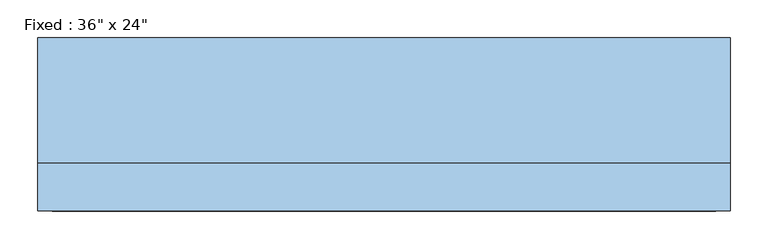
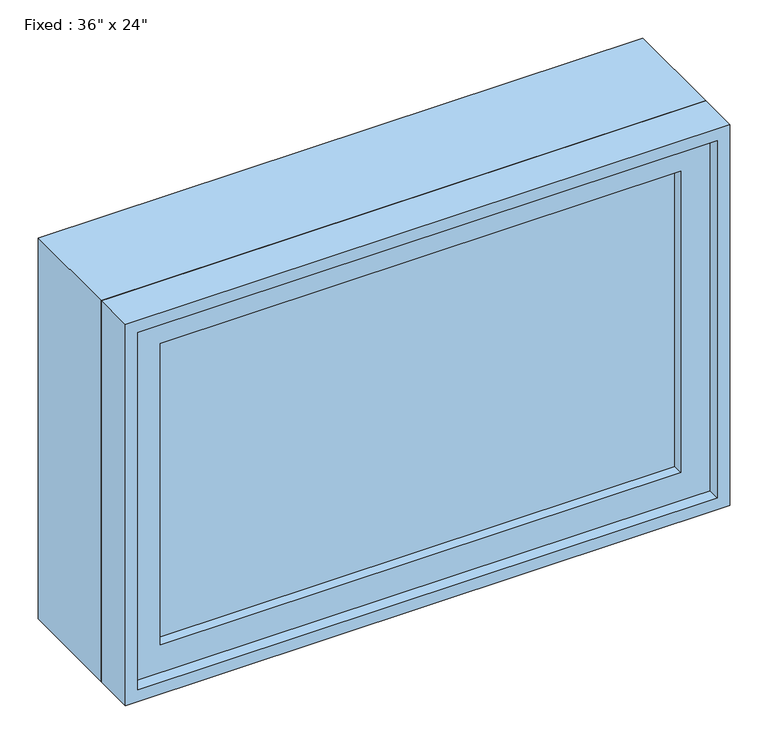
"""IFC4 building model written with IfcOpenShell, lengths in millimetres: window geometry."""

from ifc_helpers import new_model, si_unit, frame, origin, place, context, project, spatial, polyline, outline, extrude, source, transform, mapped, element, save


def window_c8489cfa(model_context):
    return source(origin(), model_context, "Body", "SweptSolid", [
        extrude(outline(polyline([(355.6, -66.675), (355.6, -79.375), (-431.8, -79.375), (-431.8, -66.675), (355.6, -66.675)])), frame((0.0, 0.0, 2197.1), z_axis=(0.0, 0.0, 1.0), x_axis=(1.0, 0.0, 0.0)), (0.0, 0.0, 1.0), 482.6),
        extrude(outline(polyline([(2724.15, -476.25), (2152.65, -476.25), (2152.65, 400.05), (2724.15, 400.05), (2724.15, -476.25)]), holes=[polyline([(2679.7, -431.8), (2679.7, 355.6), (2197.1, 355.6), (2197.1, -431.8), (2679.7, -431.8)])]), frame((0.0, -95.25, 0.0), z_axis=(0.0, 1.0, 0.0), x_axis=(0.0, 0.0, 1.0)), (0.0, 0.0, 1.0), 44.45),
        extrude(outline(polyline([(2743.2, -495.3), (2133.6, -495.3), (2133.6, 419.1), (2743.2, 419.1), (2743.2, -495.3)]), holes=[polyline([(2711.45, -463.55), (2711.45, 387.35), (2165.35, 387.35), (2165.35, -463.55), (2711.45, -463.55)])]), frame((0.0, -50.8, 0.0), z_axis=(0.0, 1.0, 0.0), x_axis=(0.0, 0.0, 1.0)), (0.0, 0.0, 1.0), 165.1),
        extrude(outline(polyline([(2743.2, 419.1), (2743.2, -495.3), (2133.6, -495.3), (2133.6, 419.1), (2743.2, 419.1)]), holes=[polyline([(2724.15, 400.05), (2152.65, 400.05), (2152.65, -476.25), (2724.15, -476.25), (2724.15, 400.05)])]), frame((0.0, -114.3, 0.0), z_axis=(0.0, 1.0, 0.0), x_axis=(0.0, 0.0, 1.0)), (0.0, 0.0, 1.0), 63.5),
    ])


if __name__ == "__main__":
    model = new_model("IFC4")
    model_context = context("Model", 3, world=origin())
    ifc_project = project(units=[si_unit("LENGTHUNIT", "METRE", prefix="MILLI")], contexts=[model_context])
    site = spatial("IfcSite", under=ifc_project)
    building = spatial("IfcBuilding", under=site)
    placement = place(None, origin())
    window_shape = window_c8489cfa(model_context)
    element("IfcWindow", 1, ObjectType="Fixed : 36\" x 24\"", at=placement, inside=building, context=model_context, shape_type="MappedRepresentation", body=[
        mapped(window_shape, transform((0.0, 0.0, 0.0), x_axis=(1.0, 0.0, 0.0), y_axis=(0.0, 1.0, 0.0), z_axis=(0.0, 0.0, 1.0))),
    ])
    save(model, "model.ifc")

# Revit data of these elements
# Type "Fixed : 36\" x 24\""
#   Type Mark = "8"
#   Construction Type Id = "GSP4R"
#   Assembly Code = "B2020100"
#   Analytic Construction = "1/8 in Pilkington single glazing"
#   Visual Light Transmittance = 0.9
#   Solar Heat Gain Coefficient = 0.78
#   Heat Transfer Coefficient (U) = 0.6496 BTU/(h·ft²·°F)
#   Height = 2' - 0"
#   Default Sill Height = 7' - 0"
#   Width = 3' - 0"
#   Window Inset = 0' - 0 3/4"
#   Define Thermal Properties by = 1
#   Define Thermal Properties by = 1
#   Glass Pane Material = Glass
#   Sash Material = Sash
#   Wall Closure = (empty or 0)
# Element 1 (IfcWindow, "Fixed : 36\" x 24\"")
#   Materials on its faces: "Sash", "Glass"
# Materials
#   "Glass": class "Glass", colour RGB 0 128 192, transparency 0.75, Description = "Soda Lime Glass", Cost = 0
#   "Sash": class "Wood", colour RGB 224 178 126, transparency 0, Cost = 0
